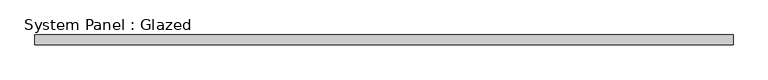
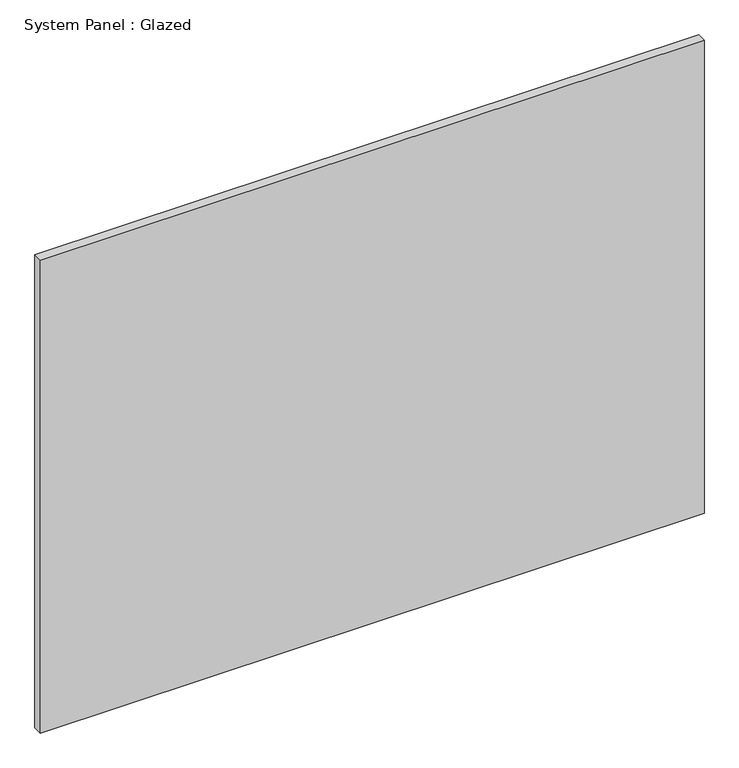
"""IFC4 building model written with IfcOpenShell, lengths in millimetres: plate geometry, System Panel : Glazed."""

from ifc_helpers import new_model, si_unit, origin, origin_with_axes, place, context, project, spatial, polyline, outline, extrude, source, transform, mapped, element, save


def system_panel_glazed_7553f7e0(model_context):
    return source(origin(), model_context, "Body", "SweptSolid", [
        extrude(outline(polyline([(912.5143734, 19.05), (-912.5143734, 19.05), (-912.5143734, 44.45), (912.5143734, 44.45), (912.5143734, 19.05)])), origin_with_axes(), (0.0, 0.0, 1.0), 1375.0426716),
    ])


if __name__ == "__main__":
    model = new_model("IFC4")
    model_context = context("Model", 3, world=origin())
    ifc_project = project(units=[si_unit("LENGTHUNIT", "METRE", prefix="MILLI")], contexts=[model_context])
    site = spatial("IfcSite", under=ifc_project)
    building = spatial("IfcBuilding", under=site)
    placement = place(None, origin())
    system_panel_glazed_shape = system_panel_glazed_7553f7e0(model_context)
    element("IfcPlate", 1, ObjectType="System Panel : Glazed", at=placement, inside=building, context=model_context, shape_type="MappedRepresentation", body=[
        mapped(system_panel_glazed_shape, transform((0.0, 0.0, 0.0), x_axis=(1.0, 0.0, 0.0), y_axis=(0.0, 1.0, 0.0), z_axis=(0.0, 0.0, 1.0))),
    ])
    save(model, "model.ifc")

# Revit data of these elements
# Type "System Panel : Glazed"
#   Construction Type Id = "GSP4R"
#   Analytic Construction = "1/8 in Pilkington single glazing"
#   Visual Light Transmittance = 0.9
#   Solar Heat Gain Coefficient = 0.86
#   Heat Transfer Coefficient (U) = 1.18115 BTU/(h·ft²·°F)
# Element 1 (IfcPlate, "System Panel : Glazed")
#   Materials on its faces: "Glass"
# Materials
#   "Glass": class "Glass", colour RGB 0 128 192, transparency 0.75, Description = "Soda Lime Glass", Cost = 0
